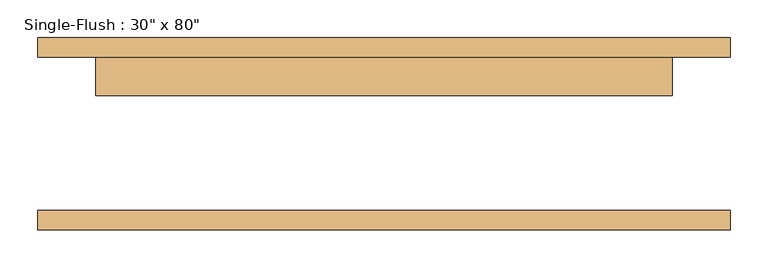
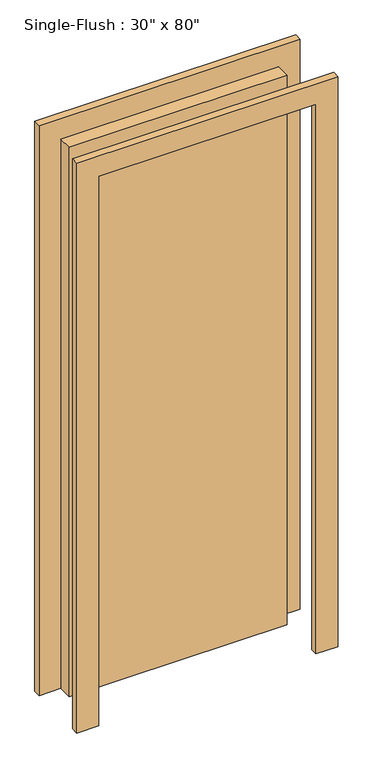
"""IFC4 building model written with IfcOpenShell, lengths in millimetres: door geometry."""

from ifc_helpers import new_model, si_unit, frame, origin, origin_with_axes, place, context, project, spatial, polyline, outline, extrude, source, transform, mapped, element, save


def door_fadea3f2(model_context):
    return source(origin(), model_context, "Body", "SweptSolid", [
        extrude(outline(polyline([(2108.2, -457.2), (0.0, -457.2), (0.0, -381.0), (2032.0, -381.0), (2032.0, 381.0), (0.0, 381.0), (0.0, 457.2), (2108.2, 457.2), (2108.2, -457.2)])), frame((0.0, 101.6, 0.0), z_axis=(0.0, 1.0, 0.0), x_axis=(0.0, 0.0, 1.0)), (0.0, 0.0, 1.0), 25.4),
        extrude(outline(polyline([(2108.2, 457.2), (2108.2, -457.2), (0.0, -457.2), (0.0, -381.0), (2032.0, -381.0), (2032.0, 381.0), (0.0, 381.0), (0.0, 457.2), (2108.2, 457.2)])), frame((0.0, -127.0, 0.0), z_axis=(0.0, 1.0, 0.0), x_axis=(0.0, 0.0, 1.0)), (0.0, 0.0, 1.0), 25.4),
        extrude(outline(polyline([(381.0, 50.8), (-381.0, 50.8), (-381.0, 101.6), (381.0, 101.6), (381.0, 50.8)])), origin_with_axes(), (0.0, 0.0, 1.0), 2032.0),
    ])


if __name__ == "__main__":
    model = new_model("IFC4")
    model_context = context("Model", 3, world=origin())
    ifc_project = project(units=[si_unit("LENGTHUNIT", "METRE", prefix="MILLI")], contexts=[model_context])
    site = spatial("IfcSite", under=ifc_project)
    building = spatial("IfcBuilding", under=site)
    placement = place(None, origin())
    door_shape = door_fadea3f2(model_context)
    element("IfcDoor", 1, ObjectType="Single-Flush : 30\" x 80\"", at=placement, inside=building, context=model_context, shape_type="MappedRepresentation", body=[
        mapped(door_shape, transform((0.0, 0.0, 0.0), x_axis=(1.0, 0.0, 0.0), y_axis=(0.0, 1.0, 0.0), z_axis=(0.0, 0.0, 1.0))),
    ])
    save(model, "model.ifc")

# Revit data of these elements
# Type "Single-Flush : 30\" x 80\""
#   Type Mark = "5"
#   Construction Type Id = "MDOOR"
#   Assembly Code = "C1020"
#   Analytic Construction = "Metal"
#   Thickness = 50.8 mm
#   Heat Transfer Coefficient (U) = 0.651978 BTU/(h·ft²·°F)
#   Height = 2032 mm
#   Trim Projection Ext = 25.4 mm
#   Trim Projection Int = 25.4 mm
#   Trim Width = 76.2 mm
#   Width = 762 mm
#   Define Thermal Properties by = 1
#   Define Thermal Properties by = 1
#   Door Material = Door - Panel
#   Frame Material = Door - Frame
#   Visual Light Transmittance = 0
#   Solar Heat Gain Coefficient = 0
#   Function = (empty or 0)
#   Wall Closure = (empty or 0)
# Element 1 (IfcDoor, "Single-Flush : 30\" x 80\"")
#   Materials on its faces: "Door - Frame", "Door - Panel"
# Materials
#   "Door - Panel": class "Wood", colour RGB 210 159 95, transparency 0, Cost = 0
#   "Door - Frame": colour RGB 118 70 51, transparency 0, Cost = 0
